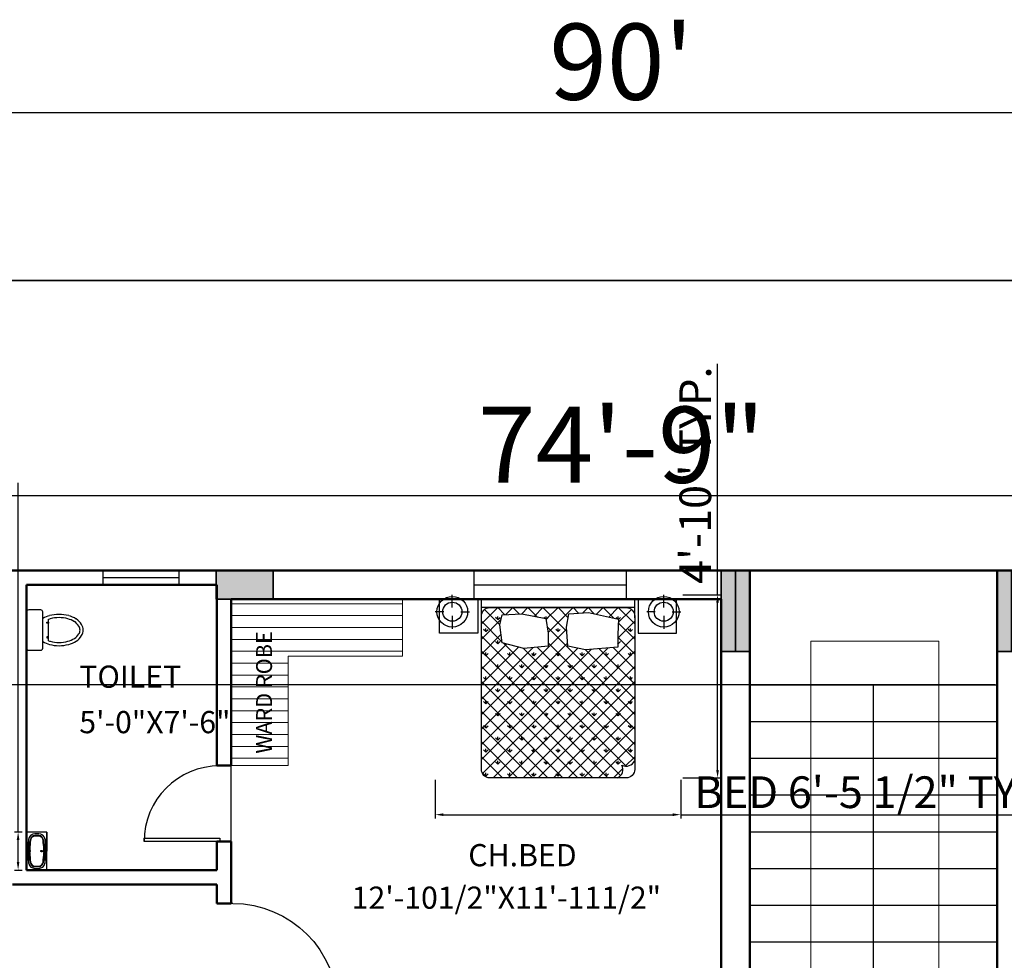
# Model space of a CAD drawing. Units: inches. Extents: x 2214 to 3937, y 762 to 2085.
# Tile 6 of 9: x 2933 to 3243, y 1789 to 2085. Entities that reach past the tile are written whole.
import ezdxf

# ---------------------------------------------------------------- set-up
doc = ezdxf.new("R2010")
doc.units = ezdxf.units.IN
for name, color, linetype, lineweight in [('A-ANNO-DIMS', 2, 'Continuous', 18), ('A-ANNO-SYMB', 6, 'Continuous', 18), ('A-ANNO-TEXT', 7, 'Continuous', 18), ('A-AREA-IDEN', 7, 'Continuous', 25), ('A-CASE-PATT', 252, 'Continuous', 13), ('A-COLS', 5, 'Continuous', 35), ('A-FLOR-FIXT', 9, 'Continuous', 18), ('A-FURN', 8, 'Continuous', 18), ('C-ANNO-DIMS', 2, 'Continuous', 18), ('C-PROP', 3, 'Continuous', 35), ('door', 122, 'Continuous', 25), ('stairs', 6, 'Continuous', 25), ('wall', 20, 'Continuous', 50), ('wardrobe', 252, 'Continuous', 18), ('window', 4, 'Continuous', 25)]:
    doc.layers.add(name, color=color, linetype=linetype, lineweight=lineweight)
for name, color, linetype in [('GIUONG', 70, 'Continuous'), ('NOI THAT', 42, 'Continuous'), ('THIET-BI', 21, 'Continuous')]:
    doc.layers.add(name, color=color, linetype=linetype)
doc.styles.get("Standard").update_dxf_attribs({"font": 'arial.ttf'})
doc.dimstyles.new('ISO-25', dxfattribs={"dimtxt": 10, "dimasz": 2.5, "dimexe": 1.25, "dimexo": 0.625, "dimtad": 1, "dimdec": 1, "dimlunit": 4, "dimtxsty": 'Standard', "dimcen": 2.5, "dimadec": 0, "dimazin": 0, "dimtfac": 1, "dimtdec": 1, "dimtmove": 0, "dimatfit": 3, "dimfxl": 1, "dimarcsym": 0})

# ---------------------------------------------------------------- blocks, each defined once
blk = doc.blocks.new('*U2')
for p, q in [((0, 0), (0, -6)), ((40, 0), (40, -6))]:
    blk.add_line(p, q)
blk.add_lwpolyline([(0, 0), (0, 40), (1.75, 40), (1.75, 0)], close=True)
blk.add_arc((0, 0), 40, 0, 90)
blk = doc.blocks.new('*X8')
at = {"color": 0}
for p, q in [((0, 0), (0, 0)), ((-707, -141), (-734, -115)), ((-707, -141), (-707, -104)), ((-707, -141), (-681, -115)), ((-566, 0), (-566, 0)), ((-566, 0), (-566, 0)), ((-283, 0), (-283, 0)), ((-283, 0), (-283, 0)), ((-156, -126), (-168, -115)), ((-141, -141), (-141, -104)), ((-141, -141), (-115, -115)), ((120, -120), (115, -115)), ((283, 0), (283, 0)), ((566, 0), (566, 0)), ((699, -134), (681, -115)), ((707, -135), (707, -104)), ((710, -139), (734, -115)), ((-141, -141), (-142, -140)), ((-849, -283), (-875, -256)), ((-849, -283), (-849, -245)), ((-849, -283), (-822, -256)), ((0, -283), (-27, -256)), ((0, -283), (0, -245)), ((0, -283), (27, -256)), ((849, -283), (822, -256)), ((849, -283), (849, -245)), ((849, -283), (875, -256)), ((-707, -424), (-734, -398)), ((-707, -424), (-707, -387)), ((-707, -424), (-681, -398)), ((-116, -399), (-115, -398)), ((707, -424), (703, -420)), ((707, -424), (707, -387)), ((707, -424), (734, -398)), ((-849, -566), (-875, -539)), ((-849, -566), (-849, -528)), ((-849, -566), (-822, -539)), ((-566, -566), (-592, -539)), ((-566, -566), (-566, -528)), ((-566, -566), (-539, -539)), ((-283, -566), (-309, -539)), ((-283, -566), (-283, -528)), ((-283, -566), (-256, -539)), ((0, -566), (-27, -539)), ((0, -566), (0, -528)), ((0, -566), (27, -539)), ((283, -566), (256, -539)), ((283, -566), (283, -528)), ((283, -566), (309, -539)), ((566, -566), (539, -539)), ((566, -566), (566, -528)), ((566, -566), (592, -539)), ((849, -566), (822, -539)), ((849, -566), (849, -528)), ((849, -566), (875, -539)), ((-707, -707), (-734, -681)), ((-707, -707), (-707, -670)), ((-707, -707), (-681, -681)), ((-424, -707), (-451, -681)), ((-424, -707), (-424, -670)), ((-424, -707), (-398, -681)), ((-141, -707), (-168, -681)), ((-141, -707), (-141, -670)), ((-141, -707), (-115, -681)), ((141, -707), (115, -681)), ((141, -707), (141, -670)), ((141, -707), (168, -681)), ((424, -707), (398, -681)), ((424, -707), (424, -670)), ((424, -707), (451, -681)), ((707, -707), (681, -681)), ((707, -707), (707, -670)), ((707, -707), (734, -681)), ((-849, -849), (-875, -822)), ((-849, -849), (-849, -811)), ((-849, -849), (-822, -822)), ((-566, -849), (-592, -822)), ((-566, -849), (-566, -811)), ((-566, -849), (-539, -822)), ((-283, -849), (-309, -822)), ((-283, -849), (-283, -811)), ((-283, -849), (-256, -822)), ((0, -849), (-27, -822)), ((0, -849), (0, -811)), ((0, -849), (27, -822)), ((283, -849), (256, -822)), ((283, -849), (283, -811)), ((283, -849), (309, -822)), ((566, -849), (539, -822)), ((566, -849), (566, -811)), ((566, -849), (592, -822)), ((849, -849), (822, -822)), ((849, -849), (849, -811)), ((849, -849), (875, -822)), ((-707, -990), (-734, -963)), ((-707, -990), (-707, -952)), ((-707, -990), (-681, -963)), ((-424, -990), (-451, -963)), ((-424, -990), (-424, -952)), ((-424, -990), (-398, -963)), ((-141, -990), (-168, -963)), ((-141, -990), (-141, -952)), ((-141, -990), (-115, -963)), ((141, -990), (115, -963)), ((141, -990), (141, -952)), ((141, -990), (168, -963)), ((424, -990), (398, -963)), ((424, -990), (424, -952)), ((424, -990), (451, -963)), ((707, -990), (681, -963)), ((707, -990), (707, -952)), ((707, -990), (734, -963)), ((-849, -1131), (-875, -1105)), ((-849, -1131), (-849, -1094)), ((-849, -1131), (-822, -1105)), ((-566, -1131), (-592, -1105)), ((-566, -1131), (-566, -1094)), ((-566, -1131), (-539, -1105)), ((-283, -1131), (-309, -1105)), ((-283, -1131), (-283, -1094)), ((-283, -1131), (-256, -1105)), ((0, -1131), (-27, -1105)), ((0, -1131), (0, -1094)), ((0, -1131), (27, -1105)), ((283, -1131), (256, -1105)), ((283, -1131), (283, -1094)), ((283, -1131), (309, -1105)), ((566, -1131), (539, -1105)), ((566, -1131), (566, -1094)), ((566, -1131), (592, -1105)), ((849, -1131), (822, -1105)), ((849, -1131), (849, -1094)), ((849, -1131), (875, -1105)), ((-707, -1273), (-734, -1246)), ((-707, -1273), (-707, -1235)), ((-707, -1273), (-681, -1246)), ((-424, -1273), (-451, -1246)), ((-424, -1273), (-424, -1235)), ((-424, -1273), (-398, -1246)), ((-141, -1273), (-168, -1246)), ((-141, -1273), (-141, -1235)), ((-141, -1273), (-115, -1246)), ((141, -1273), (115, -1246)), ((141, -1273), (141, -1235)), ((141, -1273), (168, -1246)), ((424, -1273), (398, -1246)), ((424, -1273), (424, -1235)), ((424, -1273), (451, -1246)), ((707, -1273), (681, -1246)), ((707, -1273), (707, -1235)), ((707, -1273), (734, -1246)), ((-849, -1414), (-849, -1377)), ((-566, -1414), (-566, -1377)), ((-283, -1414), (-283, -1377)), ((0, -1414), (0, -1377)), ((283, -1414), (283, -1377)), ((566, -1414), (566, -1377)), ((849, -1414), (849, -1377)), ((-849, -1414), (-875, -1388)), ((-849, -1414), (-822, -1388)), ((-566, -1414), (-592, -1388)), ((-566, -1414), (-539, -1388)), ((-283, -1414), (-309, -1388)), ((-283, -1414), (-256, -1388)), ((0, -1414), (-27, -1388)), ((0, -1414), (27, -1388)), ((283, -1414), (256, -1388)), ((283, -1414), (309, -1388)), ((566, -1414), (539, -1388)), ((566, -1414), (592, -1388)), ((849, -1414), (822, -1388)), ((849, -1414), (875, -1388)), ((-707, -1556), (-734, -1529)), ((-707, -1556), (-707, -1518)), ((-707, -1556), (-681, -1529)), ((-424, -1556), (-451, -1529)), ((-424, -1556), (-424, -1518)), ((-424, -1556), (-398, -1529)), ((-141, -1556), (-168, -1529)), ((-141, -1556), (-141, -1518)), ((-141, -1556), (-115, -1529)), ((141, -1556), (115, -1529)), ((141, -1556), (141, -1518)), ((141, -1556), (168, -1529)), ((424, -1556), (398, -1529)), ((424, -1556), (424, -1518)), ((424, -1556), (451, -1529)), ((707, -1556), (681, -1529)), ((707, -1556), (707, -1518)), ((707, -1556), (734, -1529)), ((-849, -1697), (-875, -1671)), ((-849, -1697), (-849, -1660)), ((-849, -1697), (-822, -1671)), ((-566, -1697), (-592, -1671)), ((-566, -1697), (-566, -1660)), ((-566, -1697), (-539, -1671)), ((-283, -1697), (-309, -1671)), ((-283, -1697), (-283, -1660)), ((-283, -1697), (-256, -1671)), ((0, -1697), (-27, -1671)), ((0, -1697), (0, -1660)), ((0, -1697), (27, -1671)), ((283, -1697), (256, -1671)), ((283, -1697), (283, -1660)), ((283, -1697), (309, -1671)), ((566, -1697), (539, -1671)), ((566, -1697), (566, -1660)), ((566, -1697), (592, -1671)), ((849, -1697), (822, -1671)), ((849, -1697), (849, -1660)), ((849, -1697), (875, -1671)), ((-707, -1838), (-734, -1812)), ((-707, -1838), (-707, -1801)), ((-707, -1838), (-681, -1812)), ((-424, -1838), (-451, -1812)), ((-424, -1838), (-424, -1801)), ((-424, -1838), (-398, -1812)), ((-141, -1838), (-168, -1812)), ((-141, -1838), (-141, -1801)), ((-141, -1838), (-115, -1812)), ((141, -1838), (115, -1812)), ((141, -1838), (141, -1801)), ((141, -1838), (168, -1812)), ((424, -1838), (398, -1812)), ((424, -1838), (424, -1801)), ((424, -1838), (451, -1812)), ((707, -1838), (681, -1812)), ((707, -1838), (707, -1801)), ((707, -1838), (734, -1812)), ((-849, -1980), (-875, -1953)), ((-849, -1980), (-849, -1942)), ((-849, -1980), (-822, -1953)), ((-566, -1980), (-592, -1953)), ((-566, -1980), (-566, -1942)), ((-566, -1980), (-539, -1953)), ((-283, -1980), (-309, -1953)), ((-283, -1980), (-283, -1942)), ((-283, -1980), (-256, -1953)), ((0, -1980), (-27, -1953)), ((0, -1980), (0, -1942)), ((0, -1980), (27, -1953)), ((283, -1980), (256, -1953)), ((283, -1980), (283, -1942)), ((283, -1980), (309, -1953)), ((566, -1980), (539, -1953)), ((566, -1980), (566, -1942)), ((566, -1980), (592, -1953))]:
    blk.add_line(p, q, dxfattribs=at)
blk = doc.blocks.new('*X7')
at = {"color": 0}
for p, q in [((-900, -193), (-707, 0)), ((-623, -84), (-707, 0)), ((-614, -83), (-530, 0)), ((-457, -74), (-530, 0)), ((-425, -72), (-354, 0)), ((-245, -108), (-354, 0)), ((-278, -101), (-177, 0)), ((103, -280), (-177, 0)), ((-142, -142), (0, 0)), ((-117, -294), (177, 0)), ((120, -120), (0, 0)), ((241, -64), (177, 0)), ((292, -61), (354, 0)), ((426, -72), (354, 0)), ((452, -78), (530, 0)), ((654, -123), (530, 0)), ((596, -111), (707, 0)), ((900, -193), (707, 0)), ((-683, -201), (-862, -22)), ((708, -175), (862, -22)), ((-900, -370), (-667, -137)), ((-656, -405), (-900, -161)), ((900, -1254), (-128, -225)), ((703, -358), (900, -161)), ((900, -370), (708, -178)), ((-900, -1254), (101, -252)), ((-900, -546), (-668, -314)), ((735, -1973), (-900, -337)), ((-763, -2000), (900, -337)), ((-900, -1430), (112, -418)), ((-900, -723), (-605, -429)), ((801, -1862), (-641, -419)), ((900, -1430), (-116, -415)), ((900, -546), (703, -349)), ((-900, -900), (-465, -465)), ((-900, -1077), (-293, -470)), ((-900, -1607), (231, -476)), ((-900, -1784), (394, -489)), ((586, -2000), (-900, -514)), ((-888, -1948), (586, -475)), ((-586, -2000), (900, -514)), ((900, -1784), (-404, -480)), ((900, -1607), (-243, -465)), ((900, -1077), (317, -494)), ((900, -900), (483, -483)), ((900, -723), (647, -470)), ((409, -2000), (-900, -691)), ((-409, -2000), (900, -691)), ((232, -2000), (-900, -868)), ((-232, -2000), (900, -868)), ((55, -2000), (-900, -1045)), ((-55, -2000), (900, -1045)), ((-121, -2000), (-900, -1221)), ((121, -2000), (900, -1221)), ((-298, -2000), (-900, -1398)), ((298, -2000), (900, -1398)), ((-475, -2000), (-900, -1575)), ((475, -2000), (900, -1575)), ((-652, -2000), (-900, -1752)), ((790, -1861), (900, -1752)), ((-835, -1994), (-894, -1935)), ((652, -2000), (761, -1890))]:
    blk.add_line(p, q, dxfattribs=at)
blk = doc.blocks.new('A$C190D2546')
at = {"layer": 'GIUONG'}
for points in [[(787, 1584), (758, 1799), (787, 1914), (1016, 1928), (1296, 1871), (1325, 1699), (1325, 1548), (1038, 1519)], [(1555, 1548), (1541, 1771), (1569, 1928), (1799, 1943), (2151, 1864), (2144, 1685), (2144, 1534), (1763, 1505)]]:
    blk.add_lwpolyline(points, close=True, dxfattribs=at)
for centre, radius in [((200, 1951), 180), ((2682, 1951), 180), ((200, 1951), 112), ((2682, 1951), 112)]:
    blk.add_circle(centre, radius, dxfattribs=at)
at = {"layer": 'NOI THAT'}
for p, q in [((200, 2001), (200, 2151)), ((541, 2100), (2341, 2100)), ((541, 1881), (541, 2100)), ((2341, 1881), (2341, 2100)), ((2682, 2001), (2682, 2151)), ((2341, 2000), (541, 2000)), ((100, 1951), (0, 1951)), ((200, 1901), (200, 1751)), ((300, 1951), (400, 1951)), ((2582, 1951), (2482, 1951)), ((2682, 1901), (2682, 1751)), ((2782, 1951), (2882, 1951))]:
    blk.add_line(p, q, dxfattribs=at)
for points in [[(500, 2101), (500, 1701), (50, 1701), (50, 2101)], [(2382, 2101), (2382, 1701), (2832, 1701), (2832, 2101)]]:
    blk.add_lwpolyline(points, close=True, dxfattribs=at)
blk.add_lwpolyline([(641, 2000), (2241, 2000, -0.414214), (2341, 1900), (2341, 100, -0.414214), (2241, 0), (641, 0, -0.414214), (541, 100), (541, 1900, -0.414214)], format="xyb", close=True, dxfattribs=at)
for centre, start, end in [((2091, 100), 296.5651, 26.5651), ((2241, 250), 243.4349, 333.4349)]:
    blk.add_arc(centre, 112, start, end, dxfattribs=at)
for name in ['*X7', '*X8']:
    blk.add_blockref(name, (1441, 2000), dxfattribs=at)
blk = doc.blocks.new('A$C65B13726')
at = {"layer": 'THIET-BI'}
for p, q in [((0, 400), (0, 200)), ((0, 400), (375, 400)), ((134, 362), (621, 360)), ((375, 291), (357, 291)), ((357, 291), (393, 291)), ((375, 291), (375, 309)), ((375, 309), (375, 274)), ((134, 39), (616, 39))]:
    blk.add_line(p, q, dxfattribs=at)
blk.add_lwpolyline([(0, 400), (0, 0), (750, 0), (750, 400)], close=True, dxfattribs=at)
blk.add_lwpolyline([(714, 200), (714, 240, 0.341607), (621, 360), (598, 366, 0.001439), (593, 367, 0.035276), (375, 382, 0.035276), (157, 367, 0.001439), (152, 366), (129, 360, 0.341607), (36, 240), (36, 200), (36, 161, 0.341607), (129, 40), (152, 34, 0.001439), (157, 33, 0.035276), (375, 18, 0.035276), (593, 33, 0.001439), (598, 34), (621, 40, 0.341607), (714, 161)], format="xyb", close=True, dxfattribs=at)
for points in [[(323, 348, 0.026733), (162, 334, 0.000876), (159, 333), (137, 327, 0.341782), (70, 240), (70, 161, 0.341782), (137, 73), (159, 67, 0.000876), (162, 67, 0.026747), (323, 52, 0.035276)], [(337, 337, 0.028876), (163, 323, 0.00069), (161, 322), (140, 317, 0.341861), (81, 240), (81, 160, 0.341861), (140, 83), (161, 78, 0.00069), (163, 77, 0.028898), (337, 63, 0.035276)], [(407, 348, 0.00526), (375, 349, 0.005313), (343, 348, 0.000876)], [(394, 338, 0.003179), (375, 338, 0.003179), (356, 338, 0.00069)], [(375, 382), (375, 382, 0.025118)], [(375, 382), (375, 382, 0.035276)], [(669, 200), (669, 240, 0.341861), (610, 317), (589, 322, 0.00069), (587, 323, 0.028876), (413, 337, 0.003179)], [(413, 63, 0.028961), (587, 77, 0.00069), (589, 78), (610, 83, 0.341861), (669, 160), (669, 200)], [(680, 200), (680, 240, 0.341782), (613, 327), (591, 333, 0.000876), (588, 334, 0.026733), (427, 348, 0.006503)], [(427, 52, 0.026747), (588, 67, 0.000876), (591, 67), (613, 73, 0.341782), (680, 161), (680, 200)], [(343, 52, 0.005316), (375, 52, 0.005263), (407, 52, 0.000876)], [(356, 62, 0.003135), (375, 62, 0.003135), (394, 62, 0.00069)], [(375, 17), (375, 17, 0.035276)]]:
    blk.add_lwpolyline(points, format="xyb", dxfattribs=at)
blk.add_circle((375, 291), 14.5, dxfattribs=at)
for centre, radius, start, end in [((375, 400), 73.6, 211.9576, 327.7237), ((324, 352), 19.1, 310.8832, 28.9258), ((375, 400), 65.2, 239.0852, 300.5961), ((426, 351), 19.1, 150.7555, 228.798), ((375, 0), 73.6, 32.2763, 148.0424), ((324, 48), 19.1, 331.0742, 49.1168), ((375, 0), 65.2, 59.4039, 120.9148), ((426, 49), 19.1, 131.202, 209.2445)]:
    blk.add_arc(centre, radius, start, end, dxfattribs=at)
blk = doc.blocks.new('A$C5AF77858')
at = {"layer": 'THIET-BI'}
for p, q in [((0, 675), (0, 525)), ((475, 700), (25, 700)), ((500, 525), (500, 675)), ((25, 500), (475, 500)), ((117, 430), (383, 430)), ((154, 452), (154, 430)), ((164, 452), (154, 452)), ((154, 430), (164, 430)), ((164, 430), (164, 452)), ((336, 430), (336, 452)), ((336, 452), (346, 452)), ((346, 430), (336, 430)), ((346, 452), (346, 430))]:
    blk.add_line(p, q, dxfattribs=at)
for centre, radius, start, end in [((25, 675), 25, 90, 180), ((475, 675), 25, 0, 90), ((25, 525), 25, 180, 270), ((384, 334), 323, 149.0966, 164.9269), ((116, 334), 323, 15.0731, 30.9034), ((475, 525), 25, 270, 0), ((514, 299), 458, 164.9269, 180), ((514, 299), 418, 164.9269, 180), ((384, 334), 283, 160.176, 164.9269), ((116, 334), 283, 15.0731, 19.824), ((-14, 299), 418, 0, 15.0731), ((-14, 299), 458, 0, 15.0731), ((514, 299), 458, 180, 195.0731), ((514, 299), 418, 180, 195.0731), ((-14, 299), 418, 344.9269, 0), ((-14, 299), 458, 344.9269, 0), ((384, 264), 323, 195.0731, 213.0315), ((384, 264), 283, 195.0731, 213.0315), ((116, 264), 283, 326.9685, 344.9269), ((116, 264), 323, 326.9685, 344.9269), ((302, 210), 226, 213.0315, 237.5002), ((302, 210), 186, 213.0315, 237.5002), ((250, 129), 129, 237.5002, 270), ((250, 129), 89.3, 237.5002, 270), ((250, 129), 89.3, 270, 302.4998), ((250, 129), 129, 270, 302.4998), ((198, 210), 186, 302.4998, 326.9685), ((198, 210), 226, 302.4998, 326.9685)]:
    blk.add_arc(centre, radius, start, end, dxfattribs=at)
blk = doc.blocks.new('*D19')
at = {"layer": 'C-ANNO-DIMS', "color": 0, "lineweight": -2, "ltscale": 0.3, "transparency": 16777216}
for p, q in [((2582.56, 2003.84), (2582.56, 2057.46)), ((2585.06, 2056.21), (3660.06, 2056.21)), ((3662.56, 2003.84), (3662.56, 2057.46))]:
    blk.add_line(p, q, dxfattribs=at)
at = {"layer": 'C-ANNO-DIMS', "color": 0, "ltscale": 0.3, "transparency": 16777216}
for points in [[(2585.06, 2056.63), (2585.06, 2055.8), (2582.56, 2056.21)], [(3660.06, 2056.63), (3660.06, 2055.8), (3662.56, 2056.21)]]:
    blk.add_solid(points, dxfattribs=at)
at = {"layer": 'Defpoints', "color": 0, "ltscale": 0.3, "transparency": 16777216}
for p in [(3662.56, 2056.21), (2582.56, 2003.22), (3662.56, 2003.22)]:
    blk.add_point(p, dxfattribs=at)
at = {"layer": 'C-ANNO-DIMS', "color": 0, "ltscale": 0.3, "transparency": 16777216, "insert": (3122.56, 2069.09), "char_height": 24, "attachment_point": 5}
blk.add_mtext("90'", dxfattribs=at)
blk = doc.blocks.new('*D25')
at = {"layer": 'A-ANNO-DIMS', "color": 0, "lineweight": -2, "ltscale": 0.3, "transparency": 16777216}
for p, q in [((2674.06, 1912.34), (2674.06, 1936.65)), ((2676.56, 1935.4), (3568.56, 1935.4)), ((3571.06, 1912.34), (3571.06, 1936.65))]:
    blk.add_line(p, q, dxfattribs=at)
at = {"layer": 'A-ANNO-DIMS', "color": 0, "ltscale": 0.3, "transparency": 16777216}
for points in [[(2676.56, 1935.82), (2676.56, 1934.98), (2674.06, 1935.4)], [(3568.56, 1935.82), (3568.56, 1934.98), (3571.06, 1935.4)]]:
    blk.add_solid(points, dxfattribs=at)
at = {"layer": 'Defpoints', "color": 0, "ltscale": 0.3, "transparency": 16777216}
for p in [(3571.06, 1935.4), (2674.06, 1911.72), (3571.06, 1911.72)]:
    blk.add_point(p, dxfattribs=at)
at = {"layer": 'A-ANNO-DIMS', "color": 0, "ltscale": 0.3, "transparency": 16777216, "insert": (3122.56, 1948.28), "char_height": 24, "attachment_point": 5}
blk.add_mtext('74\'-9"', dxfattribs=at)
blk = doc.blocks.new('COL-25_5X9')
at = {"ltscale": 0.3}
h = blk.add_hatch(color=256, dxfattribs=at)
h.dxf.hatch_style = 1
h.paths.add_polyline_path([(25.5, 0), (25.5, 9), (0, 9), (0, 0)])
for p, q in [((25.5, 9), (25.5, 0)), ((0, 4.5), (25.5, 4.5)), ((0, 4.5), (0, 0)), ((0, 0), (4.5, 0))]:
    blk.add_line(p, q)
blk.add_lwpolyline([(0, 9), (25.5, 9), (25.5, 0), (0, 0)], close=True, dxfattribs=at)
blk = doc.blocks.new('COL-18X9')
at = {"ltscale": 0.3}
h = blk.add_hatch(color=256, dxfattribs=at)
h.dxf.hatch_style = 1
h.paths.add_polyline_path([(18, 0), (18, 9), (0, 9), (0, 0)])
blk.add_lwpolyline([(0, 9), (18, 9), (18, 0), (0, 0)], close=True, dxfattribs=at)
blk = doc.blocks.new('WIN-48X9')
for p, q in [((0, 48), (9, 48)), ((0, 0), (9, 0))]:
    blk.add_line(p, q)
at = {"ltscale": 0.3}
blk.add_line((4.5, 0), (4.5, 48), dxfattribs=at)
blk = doc.blocks.new('WIN-24X4_5')
for p, q in [((0, 0), (0, 4.5)), ((24, 0), (24, 4.5))]:
    blk.add_line(p, q)
at = {"ltscale": 0.3}
blk.add_line((24, 2.25), (0, 2.25), dxfattribs=at)
blk = doc.blocks.new('*D45')
at = {"layer": 'C-ANNO-DIMS', "color": 0, "lineweight": -2, "ltscale": 0.3, "transparency": 16777216}
for p, q in [((3063.9, 1845.7), (3063.9, 1833.47)), ((3141.29, 1845.7), (3141.29, 1833.47)), ((3066.4, 1834.72), (3138.79, 1834.72)), ((3141.29, 1834.72), (3261.46, 1834.72))]:
    blk.add_line(p, q, dxfattribs=at)
at = {"layer": 'C-ANNO-DIMS', "color": 0, "ltscale": 0.3, "transparency": 16777216}
for points in [[(3066.4, 1835.13), (3066.4, 1834.3), (3063.9, 1834.72)], [(3138.79, 1835.13), (3138.79, 1834.3), (3141.29, 1834.72)]]:
    blk.add_solid(points, dxfattribs=at)
at = {"layer": 'Defpoints', "color": 0, "ltscale": 0.3, "transparency": 16777216}
for p in [(3063.9, 1846.33), (3141.29, 1846.33), (3141.29, 1834.72)]:
    blk.add_point(p, dxfattribs=at)
at = {"layer": 'C-ANNO-DIMS', "color": 0, "ltscale": 0.3, "transparency": 16777216, "insert": (3202.62, 1840.51), "char_height": 10, "attachment_point": 5}
blk.add_mtext('BED 6\'-5 1/2" TYP.', dxfattribs=at)
blk = doc.blocks.new('*D46')
at = {"layer": 'C-ANNO-DIMS', "color": 0, "lineweight": -2, "ltscale": 0.3, "transparency": 16777216}
for p, q in [((3152.9, 1904.08), (3152.9, 1976.96)), ((3141.91, 1904.08), (3154.15, 1904.08)), ((3152.9, 1848.83), (3152.9, 1901.58)), ((3141.91, 1846.33), (3154.15, 1846.33))]:
    blk.add_line(p, q, dxfattribs=at)
at = {"layer": 'C-ANNO-DIMS', "color": 0, "ltscale": 0.3, "transparency": 16777216}
for points in [[(3152.48, 1901.58), (3153.31, 1901.58), (3152.9, 1904.08)], [(3152.48, 1848.83), (3153.31, 1848.83), (3152.9, 1846.33)]]:
    blk.add_solid(points, dxfattribs=at)
at = {"layer": 'Defpoints', "color": 0, "ltscale": 0.3, "transparency": 16777216}
for p in [(3141.29, 1904.08), (3152.9, 1904.08), (3141.29, 1846.33)]:
    blk.add_point(p, dxfattribs=at)
at = {"layer": 'C-ANNO-DIMS', "color": 0, "ltscale": 0.3, "transparency": 16777216, "insert": (3147.16, 1941.77), "char_height": 10, "attachment_point": 5, "rotation": 90}
blk.add_mtext('4\'-10" TYP.', dxfattribs=at)
blk = doc.blocks.new('*D47')
at = {"layer": 'C-ANNO-DIMS', "color": 0, "lineweight": -2, "ltscale": 0.3, "transparency": 16777216}
for p, q in [((2932.36, 1829.27), (2932.36, 1939.34)), ((2931.18, 1829.27), (2933.61, 1829.27)), ((2932.36, 1819.77), (2932.36, 1826.77)), ((2931.18, 1817.27), (2933.61, 1817.27))]:
    blk.add_line(p, q, dxfattribs=at)
at = {"layer": 'C-ANNO-DIMS', "color": 0, "ltscale": 0.3, "transparency": 16777216}
for points in [[(2931.94, 1826.77), (2932.77, 1826.77), (2932.36, 1829.27)], [(2931.94, 1819.77), (2932.77, 1819.77), (2932.36, 1817.27)]]:
    blk.add_solid(points, dxfattribs=at)
at = {"layer": 'Defpoints', "color": 0, "ltscale": 0.3, "transparency": 16777216}
for p in [(2930.56, 1829.27), (2932.36, 1829.27), (2930.56, 1817.27)]:
    blk.add_point(p, dxfattribs=at)
at = {"layer": 'C-ANNO-DIMS', "color": 0, "ltscale": 0.3, "transparency": 16777216, "insert": (2926.56, 1885.56), "char_height": 10, "attachment_point": 5, "rotation": 90}
blk.add_mtext('BASIN 1\'-0" TYP.', dxfattribs=at)
blk = doc.blocks.new('*D62')
at = {"layer": 'C-ANNO-DIMS', "color": 0, "lineweight": -2, "ltscale": 0.3, "transparency": 16777216}
for p, q in [((3240.43, 1911.72), (2225.23, 1911.72)), ((2226.48, 1909.22), (2226.48, 1878.22)), ((3240.43, 1875.72), (2225.23, 1875.72))]:
    blk.add_line(p, q, dxfattribs=at)
at = {"layer": 'C-ANNO-DIMS', "color": 0, "ltscale": 0.3, "transparency": 16777216}
for points in [[(2226.07, 1909.22), (2226.9, 1909.22), (2226.48, 1911.72)], [(2226.07, 1878.22), (2226.9, 1878.22), (2226.48, 1875.72)]]:
    blk.add_solid(points, dxfattribs=at)
at = {"layer": 'Defpoints', "color": 0, "ltscale": 0.3, "transparency": 16777216}
for p in [(3241.06, 1911.72), (2226.48, 1875.72), (3241.06, 1875.72)]:
    blk.add_point(p, dxfattribs=at)
at = {"layer": 'C-ANNO-DIMS', "color": 0, "ltscale": 0.3, "transparency": 16777216, "insert": (2220.75, 1893.72), "char_height": 10, "attachment_point": 5, "rotation": 90}
blk.add_mtext('3\'-0"', dxfattribs=at)
blk = doc.blocks.new('*D63')
at = {"layer": 'C-ANNO-DIMS', "color": 0, "lineweight": -2, "ltscale": 0.3, "transparency": 16777216}
for p, q in [((3240.43, 1875.72), (2225.23, 1875.72)), ((2226.48, 1873.22), (2226.48, 1739.22)), ((3240.43, 1736.72), (2225.23, 1736.72))]:
    blk.add_line(p, q, dxfattribs=at)
at = {"layer": 'C-ANNO-DIMS', "color": 0, "ltscale": 0.3, "transparency": 16777216}
for points in [[(2226.07, 1873.22), (2226.9, 1873.22), (2226.48, 1875.72)], [(2226.07, 1739.22), (2226.9, 1739.22), (2226.48, 1736.72)]]:
    blk.add_solid(points, dxfattribs=at)
at = {"layer": 'Defpoints', "color": 0, "ltscale": 0.3, "transparency": 16777216}
for p in [(3241.06, 1875.72), (2226.48, 1736.72), (3241.06, 1736.72)]:
    blk.add_point(p, dxfattribs=at)
at = {"layer": 'C-ANNO-DIMS', "color": 0, "ltscale": 0.3, "transparency": 16777216, "insert": (2220.84, 1806.22), "char_height": 10, "attachment_point": 5, "rotation": 90}
blk.add_mtext('11\'-7"', dxfattribs=at)

msp = doc.modelspace()

# ---------------------------------------------------------------- hatches: boundary and pattern name
at = {"layer": 'A-CASE-PATT', "ltscale": 0.3}
h = msp.add_hatch(dxfattribs=at)
h.set_pattern_fill('ANSI31', color=256, scale=1.181102, angle=-45, style=0)
h.paths.add_polyline_path([(2999.56, 1850.22), (3017.56, 1850.22), (3017.56, 1884.72), (3053.56, 1884.72), (3053.56, 1902.72), (2999.56, 1902.72)])

# ---------------------------------------------------------------- linework, layer by layer
at = {"layer": 'A-ANNO-SYMB', "ltscale": 0.3}
for p, q in [((3182.33, 1764.86), (3182.33, 1889.49)), ((3182.33, 1889.49), (3222.71, 1889.49)), ((3222.71, 1889.49), (3222.71, 1756.48))]:
    msp.add_line(p, q, dxfattribs=at)
at = {"layer": 'C-PROP'}
msp.add_line((2582.56, 2003.22), (3662.56, 2003.22), dxfattribs=at)
at = {"layer": 'door'}
msp.add_line((2999.56, 1826.22), (2999.56, 1850.22), dxfattribs=at)
at = {"layer": 'stairs', "ltscale": 0.3}
for p, q in [((3163.06, 1875.72), (3241.06, 1875.72)), ((3202.06, 1736.72), (3202.06, 1875.72)), ((3163.06, 1864.13), (3241.06, 1864.13)), ((3163.06, 1852.54), (3241.06, 1852.54)), ((3163.06, 1840.95), (3241.06, 1840.95)), ((3163.06, 1829.36), (3241.06, 1829.36)), ((3163.06, 1817.76), (3241.06, 1817.76)), ((3163.06, 1806.17), (3241.06, 1806.17)), ((3163.06, 1794.58), (3241.06, 1794.58))]:
    msp.add_line(p, q, dxfattribs=at)
at = {"layer": 'wall'}
for p, q in [((2674.06, 1911.72), (3571.06, 1911.72)), ((3163.06, 1475.22), (3163.06, 1911.72)), ((3241.06, 1475.22), (3241.06, 1911.72)), ((2935.06, 1907.22), (2995.06, 1907.22)), ((2935.06, 1817.22), (2935.06, 1907.22)), ((2995.06, 1850.22), (2995.06, 1907.22)), ((2999.56, 1902.72), (3154.06, 1902.72)), ((2999.56, 1850.22), (2999.56, 1902.72)), ((3154.06, 1769.22), (3154.06, 1902.72)), ((2995.06, 1850.22), (2999.56, 1850.22)), ((2995.06, 1817.22), (2995.06, 1826.22)), ((2995.06, 1826.22), (2999.56, 1826.22)), ((2999.56, 1806.72), (2999.56, 1826.22)), ((2935.06, 1817.22), (2995.06, 1817.22)), ((2930.56, 1812.72), (2995.06, 1812.72)), ((2995.06, 1806.72), (2995.06, 1812.72)), ((2995.06, 1806.72), (2999.56, 1806.72))]:
    msp.add_line(p, q, dxfattribs=at)
at = {"layer": 'wardrobe'}
for p, q in [((3053.56, 1884.72), (3053.56, 1902.72)), ((3017.56, 1850.22), (3017.56, 1884.72)), ((3017.56, 1884.72), (3053.56, 1884.72)), ((2999.56, 1850.22), (3017.56, 1850.22))]:
    msp.add_line(p, q, dxfattribs=at)

# ---------------------------------------------------------------- block references
at = {"layer": 'A-COLS'}
msp.add_blockref('COL-18X9', (2994.83, 1902.72), dxfattribs=at)
at = {"layer": 'A-COLS', "rotation": 269.9999999999964}
for p in [(3154.06, 1911.72), (3241.06, 1911.72)]:
    msp.add_blockref('COL-25_5X9', p, dxfattribs=at)
at = {"layer": 'A-FLOR-FIXT'}
for name, p, xscale, yscale, zscale, rotation in [('A$C5AF77858', (2952.89, 1886.58), 0.0254713121376822, 0.0254713121376822, 0.0254713121376822, 90), ('A$C65B13726', (2935.06, 1829.22), 0.0160009442456078, 0.0160009442456078, 0.0160009442456078, 270)]:
    msp.add_blockref(name, p, dxfattribs=dict(at, xscale=xscale, yscale=yscale, zscale=zscale, rotation=rotation))
at = {"layer": 'A-FURN', "xscale": 0.0268541596481872, "yscale": 0.0268541596481872, "zscale": 0.0268541596481872}
msp.add_blockref('A$C190D2546', (3063.9, 1846.33), dxfattribs=at)
at = {"layer": 'door'}
for p, xscale, yscale, zscale, rotation in [((2995.97, 1826.22), 0.5977483086185204, 0.5977483086185204, 0.5977483086185204, 90), ((3000.02, 1773.63), -0.8273413149108705, 0.8273413149108705, 0.8273413149108705, 270)]:
    msp.add_blockref('*U2', p, dxfattribs=dict(at, xscale=xscale, yscale=yscale, zscale=zscale, rotation=rotation))
at = {"layer": 'window'}
for name, p, rotation in [('WIN-24X4_5', (2983.06, 1911.72), 180), ('WIN-48X9', (3076.06, 1911.72), 270.0000000000023)]:
    msp.add_blockref(name, p, dxfattribs=dict(at, rotation=rotation))

# ---------------------------------------------------------------- texts
at = {"layer": 'A-ANNO-TEXT', "ltscale": 0.3}
msp.add_text('WARD ROBE', height=5, rotation=90, dxfattribs=at).set_placement((3012.41, 1853.97))
at = {"layer": 'A-AREA-IDEN', "ltscale": 0.3}
for s, p in [('TOILET', (2951.65, 1874.74)), ('5\'-0"X7\'-6"', (2951.65, 1860.41)), ('CH.BED', (3074.3, 1818.45)), ('12\'-101/2"X11\'-111/2"', (3037.53, 1805.04))]:
    msp.add_text(s, height=7, dxfattribs=at).set_placement(p)

# ---------------------------------------------------------------- dimensions: what is measured, and where the dimension line sits
at = {"layer": 'A-ANNO-DIMS', "ltscale": 0.3}
dim = msp.add_linear_dim(base=(3571.06, 1935.4), p1=(2674.06, 1911.72), p2=(3571.06, 1911.72), dimstyle='ISO-25', override={"dimtxt": 24, "dimclrd": 0, "dimclre": 0, "dimclrt": 0}, dxfattribs=at)
dim.commit()
dim.dimension.update_dxf_attribs({"geometry": '*D25', "text_midpoint": (3122.56, 1948.28)})
at = {"layer": 'C-ANNO-DIMS', "ltscale": 0.3}
dim = msp.add_linear_dim(base=(3662.56, 2056.21), p1=(2582.56, 2003.22), p2=(3662.56, 2003.22), dimstyle='ISO-25', override={"dimtxt": 24, "dimclrd": 0, "dimclre": 0, "dimclrt": 0}, dxfattribs=at)
dim.commit()
dim.dimension.update_dxf_attribs({"geometry": '*D19', "text_midpoint": (3122.56, 2069.09)})
for base, p1, p2, text, picture, middle in [((3152.8953, 1904.0804), (3141.2871, 1846.3252), (3141.2871, 1904.0804), '<> TYP.', '*D46', (3147.1646, 1941.7689)), ((2932.36, 1829.27), (2930.56, 1817.27), (2930.56, 1829.27), 'BASIN <> TYP.', '*D47', (2926.56, 1885.56))]:
    dim = msp.add_linear_dim(base=base, p1=p1, p2=p2, angle=90, text=text, dimstyle='ISO-25', override={"dimdec": 1, "dimlfac": 1, "dimrnd": 0, "dimzin": 1, "dimdsep": 46, "dimlunit": 4, "dimfrac": 2}, dxfattribs=at)
    dim.commit()
    dim.dimension.update_dxf_attribs({"geometry": picture, "text_midpoint": middle})
for base, p1, p2, picture, middle in [((2226.48, 1875.72), (3241.06, 1911.72), (3241.06, 1875.72), '*D62', (2220.75, 1893.72)), ((2226.48, 1736.72), (3241.06, 1875.72), (3241.06, 1736.72), '*D63', (2220.84, 1806.22))]:
    dim = msp.add_linear_dim(base=base, p1=p1, p2=p2, angle=90, dimstyle='ISO-25', override={"dimdec": 1, "dimlfac": 1, "dimrnd": 0, "dimzin": 1, "dimdsep": 46, "dimlunit": 4, "dimfrac": 2}, dxfattribs=at)
    dim.commit()
    dim.dimension.update_dxf_attribs({"geometry": picture, "text_midpoint": middle})
dim = msp.add_linear_dim(base=(3141.29, 1834.72), p1=(3063.9, 1846.33), p2=(3141.29, 1846.33), text='BED <> TYP.', dimstyle='ISO-25', override={"dimdec": 1, "dimlfac": 1, "dimrnd": 0, "dimzin": 1, "dimdsep": 46, "dimlunit": 4, "dimfrac": 2}, dxfattribs=at)
dim.commit()
dim.dimension.update_dxf_attribs({"geometry": '*D45', "text_midpoint": (3202.62, 1840.51)})

doc.saveas('drawing.dxf')
